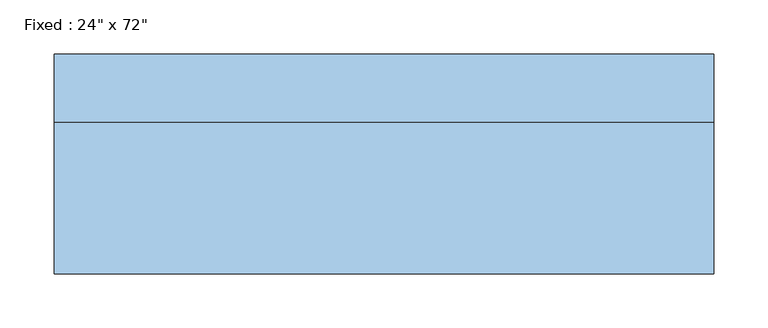
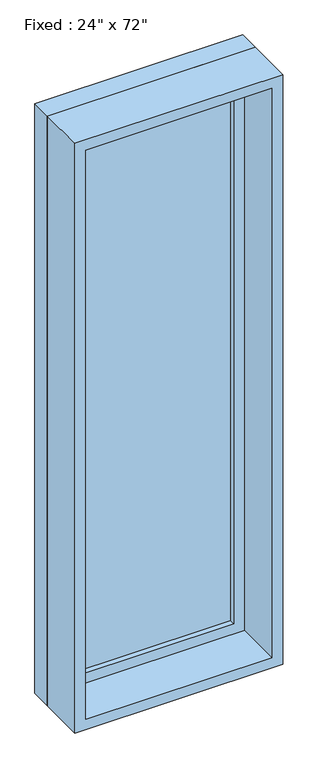
"""IFC4 building model written with IfcOpenShell, lengths in millimetres: window geometry."""

from ifc_helpers import new_model, si_unit, frame, origin, place, context, project, spatial, polyline, outline, extrude, source, transform, mapped, element, save


def window_50feeedf(model_context):
    return source(origin(), model_context, "Body", "SweptSolid", [
        extrude(outline(polyline([(203.2, 53.975), (-279.4, 53.975), (-279.4, 66.675), (203.2, 66.675), (203.2, 53.975)])), frame((0.0, 0.0, 368.3), z_axis=(0.0, 0.0, 1.0), x_axis=(1.0, 0.0, 0.0)), (0.0, 0.0, 1.0), 1701.8),
        extrude(outline(polyline([(2114.55, -323.85), (323.85, -323.85), (323.85, 247.65), (2114.55, 247.65), (2114.55, -323.85)]), holes=[polyline([(2070.1, -279.4), (2070.1, 203.2), (368.3, 203.2), (368.3, -279.4), (2070.1, -279.4)])]), frame((0.0, 38.1, 0.0), z_axis=(0.0, 1.0, 0.0), x_axis=(0.0, 0.0, 1.0)), (0.0, 0.0, 1.0), 44.45),
        extrude(outline(polyline([(2133.6, -342.9), (304.8, -342.9), (304.8, 266.7), (2133.6, 266.7), (2133.6, -342.9)]), holes=[polyline([(2101.85, -311.15), (2101.85, 234.95), (336.55, 234.95), (336.55, -311.15), (2101.85, -311.15)])]), frame((0.0, -101.6, 0.0), z_axis=(0.0, 1.0, 0.0), x_axis=(0.0, 0.0, 1.0)), (0.0, 0.0, 1.0), 139.7),
        extrude(outline(polyline([(2133.6, 266.7), (2133.6, -342.9), (304.8, -342.9), (304.8, 266.7), (2133.6, 266.7)]), holes=[polyline([(2114.55, 247.65), (323.85, 247.65), (323.85, -323.85), (2114.55, -323.85), (2114.55, 247.65)])]), frame((0.0, 38.1, 0.0), z_axis=(0.0, 1.0, 0.0), x_axis=(0.0, 0.0, 1.0)), (0.0, 0.0, 1.0), 63.5),
    ])


if __name__ == "__main__":
    model = new_model("IFC4")
    model_context = context("Model", 3, world=origin())
    ifc_project = project(units=[si_unit("LENGTHUNIT", "METRE", prefix="MILLI")], contexts=[model_context])
    site = spatial("IfcSite", under=ifc_project)
    building = spatial("IfcBuilding", under=site)
    placement = place(None, origin())
    window_shape = window_50feeedf(model_context)
    element("IfcWindow", 1, ObjectType="Fixed : 24\" x 72\"", at=placement, inside=building, context=model_context, shape_type="MappedRepresentation", body=[
        mapped(window_shape, transform((0.0, 0.0, 0.0), x_axis=(1.0, 0.0, 0.0), y_axis=(0.0, 1.0, 0.0), z_axis=(0.0, 0.0, 1.0))),
    ])
    save(model, "model.ifc")

# Revit data of these elements
# Type "Fixed : 24\" x 72\""
#   Type Mark = "7"
#   Construction Type Id = "GSP4R"
#   Assembly Code = "B2020100"
#   Analytic Construction = "1/8 in Pilkington single glazing"
#   Visual Light Transmittance = 0.9
#   Solar Heat Gain Coefficient = 0.78
#   Heat Transfer Coefficient (U) = 0.6496 BTU/(h·ft²·°F)
#   Height = 6' - 0"
#   Default Sill Height = 1' - 0"
#   Width = 2' - 0"
#   Window Inset = 0' - 0 3/4"
#   Define Thermal Properties by = 1
#   Glass Pane Material = Glass
#   Sash Material = Sash
#   Wall Closure = (empty or 0)
# Element 1 (IfcWindow, "Fixed : 24\" x 72\"")
#   Materials on its faces: "Sash", "Glass"
# Materials
#   "Glass": class "Glass", colour RGB 0 128 192, transparency 0.75, Description = "Soda Lime Glass", Cost = 0
#   "Sash": class "Wood", colour RGB 224 178 126, transparency 0
